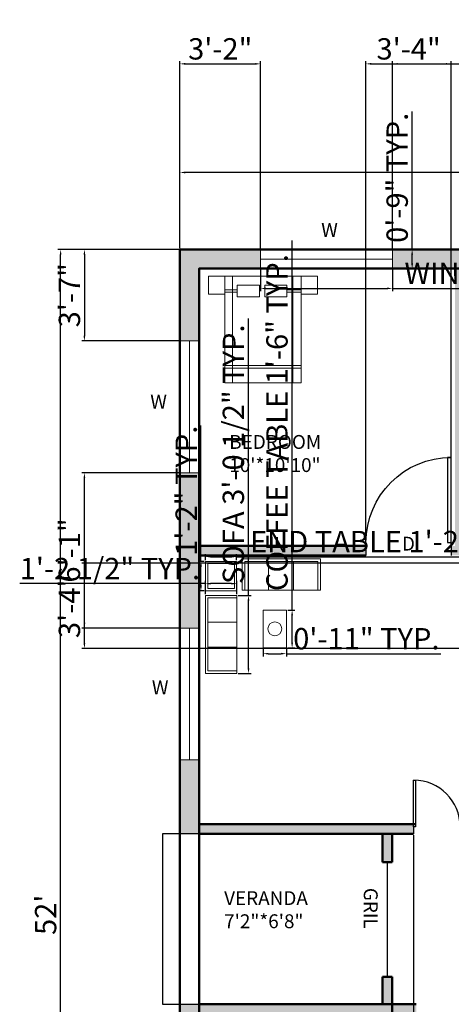
# Model space of a CAD drawing. Units: inches. Extents: x 1935 to 2445, y 1978 to 2806.
# Tile 2 of 4: x 1935 to 2137, y 2344 to 2806. Entities that reach past the tile are written whole.
import ezdxf

# ---------------------------------------------------------------- set-up
doc = ezdxf.new("R2010")
doc.units = ezdxf.units.IN
for name, color, linetype, lineweight in [('A-ANNO-DIMS', 2, 'Continuous', 18), ('A-ANNO-TEXT', 7, 'Continuous', 25), ('A-AREA-IDEN', 130, 'Continuous', 25), ('A-DOOR', 3, 'Continuous', 25), ('A-FLOR-GRIL', 3, 'Continuous', 25), ('A-FLOR-OTLN', 7, 'Continuous', 25), ('A-FURN', 9, 'Continuous', 18), ('A-GLAZ', 4, 'Continuous', 18), ('A-WALL-PATT', 225, 'Continuous', 13), ('SOFA', 10, 'Continuous', 18), ('WALL', 225, 'Continuous', 50)]:
    doc.layers.add(name, color=color, linetype=linetype, lineweight=lineweight)
doc.styles.get("Standard").update_dxf_attribs({"font": 'arial.ttf'})
doc.dimstyles.new('ISO-25', dxfattribs={"dimtxt": 10, "dimasz": 2.5, "dimexe": 1.25, "dimexo": 0.625, "dimtad": 1, "dimdec": 0, "dimlunit": 4, "dimtxsty": 'Standard', "dimcen": 2.5, "dimadec": 0, "dimazin": 0, "dimtfac": 1, "dimtdec": 0, "dimtmove": 0, "dimatfit": 3, "dimfxl": 1, "dimarcsym": 0})

# ---------------------------------------------------------------- blocks, each defined once
blk = doc.blocks.new('*U2')
for p, q in [((0, 0), (0, -6)), ((40, 0), (40, -6))]:
    blk.add_line(p, q)
blk.add_lwpolyline([(0, 0), (0, 40), (1.75, 40), (1.75, 0)], close=True)
blk.add_arc((0, 0), 40, 0, 90)
blk = doc.blocks.new('*D8')
at = {"layer": 'A-ANNO-DIMS', "color": 0, "lineweight": -2, "transparency": 16777216}
for p, q in [((2010.18, 2698.51), (2010.18, 2735.24)), ((2331.68, 2733.99), (2012.68, 2733.99)), ((2334.18, 2698.51), (2334.18, 2735.24))]:
    blk.add_line(p, q, dxfattribs=at)
at = {"layer": 'A-ANNO-DIMS', "color": 0, "lineweight": 100, "transparency": 16777216}
for points in [[(2012.68, 2734.4), (2012.68, 2733.57), (2010.18, 2733.99)], [(2331.68, 2734.4), (2331.68, 2733.57), (2334.18, 2733.99)]]:
    blk.add_solid(points, dxfattribs=at)
at = {"layer": 'Defpoints', "color": 0, "lineweight": 100, "transparency": 16777216}
for p in [(2010.18, 2733.99), (2010.18, 2697.88), (2334.18, 2697.88)]:
    blk.add_point(p, dxfattribs=at)
at = {"layer": 'A-ANNO-DIMS', "color": 0, "transparency": 16777216, "insert": (2172.18, 2739.63), "char_height": 10, "attachment_point": 5}
blk.add_mtext("27'", dxfattribs=at)
blk = doc.blocks.new('*D9')
at = {"layer": 'A-ANNO-DIMS', "color": 0, "lineweight": -2, "transparency": 16777216}
for p, q in [((2333.56, 2697.88), (1952.98, 2697.88)), ((1954.23, 2076.38), (1954.23, 2695.38)), ((2333.56, 2073.88), (1952.98, 2073.88))]:
    blk.add_line(p, q, dxfattribs=at)
at = {"layer": 'A-ANNO-DIMS', "color": 0, "lineweight": 100, "transparency": 16777216}
for points in [[(1953.82, 2695.38), (1954.65, 2695.38), (1954.23, 2697.88)], [(1953.82, 2076.38), (1954.65, 2076.38), (1954.23, 2073.88)]]:
    blk.add_solid(points, dxfattribs=at)
at = {"layer": 'Defpoints', "color": 0, "lineweight": 100, "transparency": 16777216}
for p in [(1954.23, 2697.88), (2334.18, 2697.88), (2334.18, 2073.88)]:
    blk.add_point(p, dxfattribs=at)
at = {"layer": 'A-ANNO-DIMS', "color": 0, "transparency": 16777216, "insert": (1948.5, 2385.88), "char_height": 10, "attachment_point": 5, "rotation": 90}
blk.add_mtext("52'", dxfattribs=at)
blk = doc.blocks.new('WINDOW-STD')
blk.add_line((0, 4.5), (61.82, 4.5))
blk.add_lwpolyline([(0, 9), (61.82, 9), (61.82, 0), (0, 0)], close=True)
blk = doc.blocks.new('BED-WITH-NIGHTSTANDS')
for p, q in [((11.32, 50.11), (11.32, 0)), ((39.64, 0), (39.64, 50.11)), ((13.46, 43.65), (7.73, 43.65)), ((13.46, 42.6), (7.73, 42.6)), ((43.47, 43.65), (36.85, 43.65)), ((43.47, 42.6), (36.85, 42.6)), ((7.73, 8.18), (43.47, 8.18)), ((7.73, 6.93), (43.47, 6.93)), ((43.47, 0), (39.64, 0))]:
    blk.add_line(p, q)
for points in [[(0, 50.11), (7.73, 50.11), (7.73, 41.64), (0, 41.64)], [(7.73, 50.11), (43.47, 50.11), (43.47, 0), (7.73, 0)], [(43.47, 50.11), (51.2, 50.11), (51.2, 41.64), (43.47, 41.64)], [(13.46, 45.91), (23.93, 45.91), (23.93, 40.33), (13.46, 40.33)], [(26.4, 45.91), (36.86, 45.91), (36.86, 40.33), (26.4, 40.33)]]:
    blk.add_lwpolyline(points, close=True)
blk = doc.blocks.new('SOFA-3-SEAT')
for p, q in [((0, 0), (0, 14.72)), ((0, 14.72), (36.65, 14.72)), ((36.65, 14.72), (36.65, 0)), ((12.37, 13.53), (12.37, 0)), ((24.09, 13.53), (24.09, 0)), ((1.26, 0), (0, 0)), ((36.65, 0), (31.67, 0))]:
    blk.add_line(p, q)
blk.add_lwpolyline([(1.26, 0), (35.43, 0), (35.43, 13.53), (1.26, 13.53)], close=True)
blk = doc.blocks.new('TABLE-END')
for points in [[(0, 13.76), (14.51, 13.76), (14.51, 0), (0, 0)], [(1, 12.76), (13.51, 12.76), (13.51, 1), (1, 1)]]:
    blk.add_lwpolyline(points, close=True)
blk = doc.blocks.new('TABLE-COFFEE')
blk.add_lwpolyline([(0, 0), (10.92, 0), (10.92, 17.81), (0, 17.81)], close=True)
blk.add_circle((5.5, 9), 3.27)
blk = doc.blocks.new('*D18')
at = {"layer": 'A-ANNO-DIMS', "color": 0, "lineweight": -2, "transparency": 16777216}
for p, q in [((2047.95, 2688.26), (2047.95, 2678.36)), ((2109.77, 2688.26), (2109.77, 2678.36)), ((2050.45, 2679.61), (2107.27, 2679.61)), ((2109.77, 2679.61), (2240.06, 2679.61))]:
    blk.add_line(p, q, dxfattribs=at)
at = {"layer": 'A-ANNO-DIMS', "color": 0, "lineweight": 100, "transparency": 16777216}
for points in [[(2050.45, 2680.03), (2050.45, 2679.19), (2047.95, 2679.61)], [(2107.27, 2680.03), (2107.27, 2679.19), (2109.77, 2679.61)]]:
    blk.add_solid(points, dxfattribs=at)
at = {"layer": 'Defpoints', "color": 0, "lineweight": 100, "transparency": 16777216}
for p in [(2047.95, 2688.88), (2109.77, 2688.88), (2109.77, 2679.61)]:
    blk.add_point(p, dxfattribs=at)
at = {"layer": 'A-ANNO-DIMS', "color": 0, "transparency": 16777216, "insert": (2176.16, 2685.41), "char_height": 10, "attachment_point": 5}
blk.add_mtext('WINDOW 5\'-2" TYP.', dxfattribs=at)
blk = doc.blocks.new('*D19')
at = {"layer": 'A-ANNO-DIMS', "color": 0, "lineweight": -2, "transparency": 16777216}
for p, q in [((2119.04, 2697.88), (2119.04, 2762.59)), ((2110.39, 2697.88), (2120.29, 2697.88)), ((2119.04, 2691.38), (2119.04, 2695.38)), ((2110.39, 2688.88), (2120.29, 2688.88))]:
    blk.add_line(p, q, dxfattribs=at)
at = {"layer": 'A-ANNO-DIMS', "color": 0, "lineweight": 100, "transparency": 16777216}
for points in [[(2118.62, 2695.38), (2119.46, 2695.38), (2119.04, 2697.88)], [(2118.62, 2691.38), (2119.46, 2691.38), (2119.04, 2688.88)]]:
    blk.add_solid(points, dxfattribs=at)
at = {"layer": 'Defpoints', "color": 0, "lineweight": 100, "transparency": 16777216}
for p in [(2109.77, 2697.88), (2119.04, 2697.88), (2109.77, 2688.88)]:
    blk.add_point(p, dxfattribs=at)
at = {"layer": 'A-ANNO-DIMS', "color": 0, "transparency": 16777216, "insert": (2113.31, 2731.49), "char_height": 10, "attachment_point": 5, "rotation": 90}
blk.add_mtext('0\'-9" TYP.', dxfattribs=at)
blk = doc.blocks.new('*D24')
at = {"layer": 'A-ANNO-DIMS', "color": 0, "lineweight": -2, "transparency": 16777216}
for p, q in [((2042.32, 2535.66), (2042.32, 2665.53)), ((2037.44, 2535.66), (2043.57, 2535.66)), ((2042.32, 2501.51), (2042.32, 2533.16)), ((2037.44, 2499.01), (2043.57, 2499.01))]:
    blk.add_line(p, q, dxfattribs=at)
at = {"layer": 'A-ANNO-DIMS', "color": 0, "lineweight": 100, "transparency": 16777216}
for points in [[(2041.9, 2533.16), (2042.73, 2533.16), (2042.32, 2535.66)], [(2041.9, 2501.51), (2042.73, 2501.51), (2042.32, 2499.01)]]:
    blk.add_solid(points, dxfattribs=at)
at = {"layer": 'Defpoints', "color": 0, "lineweight": 100, "transparency": 16777216}
for p in [(2036.82, 2535.66), (2042.32, 2535.66), (2036.82, 2499.01)]:
    blk.add_point(p, dxfattribs=at)
at = {"layer": 'A-ANNO-DIMS', "color": 0, "transparency": 16777216, "insert": (2036.51, 2601.85), "char_height": 10, "attachment_point": 5, "rotation": 90}
blk.add_mtext('SOFA 3\'-0 1/2" TYP.', dxfattribs=at)
blk = doc.blocks.new('*D25')
at = {"layer": 'A-ANNO-DIMS', "color": 0, "lineweight": -2, "transparency": 16777216}
for p, q in [((2022.1, 2541.16), (1935.04, 2541.16)), ((2022.1, 2536.28), (2022.1, 2542.41)), ((2034.32, 2541.16), (2024.6, 2541.16)), ((2036.82, 2536.28), (2036.82, 2542.41))]:
    blk.add_line(p, q, dxfattribs=at)
at = {"layer": 'A-ANNO-DIMS', "color": 0, "lineweight": 100, "transparency": 16777216}
for points in [[(2024.6, 2541.57), (2024.6, 2540.74), (2022.1, 2541.16)], [(2034.32, 2541.57), (2034.32, 2540.74), (2036.82, 2541.16)]]:
    blk.add_solid(points, dxfattribs=at)
at = {"layer": 'Defpoints', "color": 0, "lineweight": 100, "transparency": 16777216}
for p in [(2022.1, 2541.16), (2022.1, 2535.66), (2036.82, 2535.66)]:
    blk.add_point(p, dxfattribs=at)
at = {"layer": 'A-ANNO-DIMS', "color": 0, "transparency": 16777216, "insert": (1977.32, 2546.95), "char_height": 10, "attachment_point": 5}
blk.add_mtext('1\'-2 1/2" TYP.', dxfattribs=at)
blk = doc.blocks.new('*D26')
at = {"layer": 'A-ANNO-DIMS', "color": 0, "lineweight": -2, "transparency": 16777216}
for p, q in [((2022.21, 2552.24), (2022.21, 2555.04)), ((2024.71, 2553.79), (2034.22, 2553.79)), ((2036.72, 2552.24), (2036.72, 2555.04)), ((2036.72, 2553.79), (2205.72, 2553.79))]:
    blk.add_line(p, q, dxfattribs=at)
at = {"layer": 'A-ANNO-DIMS', "color": 0, "lineweight": 100, "transparency": 16777216}
for points in [[(2024.71, 2554.21), (2024.71, 2553.37), (2022.21, 2553.79)], [(2034.22, 2554.21), (2034.22, 2553.37), (2036.72, 2553.79)]]:
    blk.add_solid(points, dxfattribs=at)
at = {"layer": 'Defpoints', "color": 0, "lineweight": 100, "transparency": 16777216}
for p in [(2036.72, 2553.79), (2022.21, 2551.61), (2036.72, 2551.61)]:
    blk.add_point(p, dxfattribs=at)
at = {"layer": 'A-ANNO-DIMS', "color": 0, "transparency": 16777216, "insert": (2122.47, 2559.59), "char_height": 10, "attachment_point": 5}
blk.add_mtext('END TABLE 1\'-2 1/2" TYP.', dxfattribs=at)
blk = doc.blocks.new('*D27')
at = {"layer": 'A-ANNO-DIMS', "color": 0, "lineweight": -2, "transparency": 16777216}
for p, q in [((2020.04, 2551.61), (2020.04, 2615.38)), ((2021.59, 2551.61), (2018.79, 2551.61)), ((2020.04, 2540.35), (2020.04, 2549.11)), ((2021.59, 2537.85), (2018.79, 2537.85))]:
    blk.add_line(p, q, dxfattribs=at)
at = {"layer": 'A-ANNO-DIMS', "color": 0, "lineweight": 100, "transparency": 16777216}
for points in [[(2019.62, 2549.11), (2020.46, 2549.11), (2020.04, 2551.61)], [(2019.62, 2540.35), (2020.46, 2540.35), (2020.04, 2537.85)]]:
    blk.add_solid(points, dxfattribs=at)
at = {"layer": 'Defpoints', "color": 0, "lineweight": 100, "transparency": 16777216}
for p in [(2020.04, 2551.61), (2022.21, 2551.61), (2022.21, 2537.85)]:
    blk.add_point(p, dxfattribs=at)
at = {"layer": 'A-ANNO-DIMS', "color": 0, "transparency": 16777216, "insert": (2014.39, 2584.75), "char_height": 10, "attachment_point": 5, "rotation": 90}
blk.add_mtext('1\'-2" TYP.', dxfattribs=at)
blk = doc.blocks.new('*D28')
at = {"layer": 'A-ANNO-DIMS', "color": 0, "lineweight": -2, "transparency": 16777216}
for p, q in [((2062.76, 2528.8), (2062.76, 2702.06)), ((2060.71, 2528.8), (2064.01, 2528.8)), ((2062.76, 2513.49), (2062.76, 2526.3)), ((2060.71, 2510.99), (2064.01, 2510.99))]:
    blk.add_line(p, q, dxfattribs=at)
at = {"layer": 'A-ANNO-DIMS', "color": 0, "lineweight": 100, "transparency": 16777216}
for points in [[(2062.34, 2526.3), (2063.17, 2526.3), (2062.76, 2528.8)], [(2062.34, 2513.49), (2063.17, 2513.49), (2062.76, 2510.99)]]:
    blk.add_solid(points, dxfattribs=at)
at = {"layer": 'Defpoints', "color": 0, "lineweight": 100, "transparency": 16777216}
for p in [(2060.08, 2528.8), (2062.76, 2528.8), (2060.08, 2510.99)]:
    blk.add_point(p, dxfattribs=at)
at = {"layer": 'A-ANNO-DIMS', "color": 0, "transparency": 16777216, "insert": (2056.96, 2616.68), "char_height": 10, "attachment_point": 5, "rotation": 90}
blk.add_mtext('COFFEE TABLE 1\'-6" TYP.', dxfattribs=at)
blk = doc.blocks.new('*D29')
at = {"layer": 'A-ANNO-DIMS', "color": 0, "lineweight": -2, "transparency": 16777216}
for p, q in [((2049.17, 2510.36), (2049.17, 2507.07)), ((2051.67, 2508.32), (2057.58, 2508.32)), ((2060.08, 2510.36), (2060.08, 2507.07)), ((2060.08, 2508.32), (2132.56, 2508.32))]:
    blk.add_line(p, q, dxfattribs=at)
at = {"layer": 'A-ANNO-DIMS', "color": 0, "lineweight": 100, "transparency": 16777216}
for points in [[(2051.67, 2508.73), (2051.67, 2507.9), (2049.17, 2508.32)], [(2057.58, 2508.73), (2057.58, 2507.9), (2060.08, 2508.32)]]:
    blk.add_solid(points, dxfattribs=at)
at = {"layer": 'Defpoints', "color": 0, "lineweight": 100, "transparency": 16777216}
for p in [(2049.17, 2510.99), (2060.08, 2510.99), (2060.08, 2508.32)]:
    blk.add_point(p, dxfattribs=at)
at = {"layer": 'A-ANNO-DIMS', "color": 0, "transparency": 16777216, "insert": (2097.57, 2514.05), "char_height": 10, "attachment_point": 5}
blk.add_mtext('0\'-11" TYP.', dxfattribs=at)
blk = doc.blocks.new('*D34')
at = {"layer": 'A-ANNO-DIMS', "color": 0, "lineweight": -2, "transparency": 16777216}
for p, q in [((2010.18, 2698.51), (2010.18, 2786.17)), ((2012.68, 2784.92), (2045.45, 2784.92)), ((2047.95, 2698.51), (2047.95, 2786.17))]:
    blk.add_line(p, q, dxfattribs=at)
at = {"layer": 'A-ANNO-DIMS', "color": 0, "lineweight": 100, "transparency": 16777216}
for points in [[(2012.68, 2785.34), (2012.68, 2784.51), (2010.18, 2784.92)], [(2045.45, 2785.34), (2045.45, 2784.51), (2047.95, 2784.92)]]:
    blk.add_solid(points, dxfattribs=at)
at = {"layer": 'Defpoints', "color": 0, "lineweight": 100, "transparency": 16777216}
for p in [(2047.95, 2784.92), (2010.18, 2697.88), (2047.95, 2697.88)]:
    blk.add_point(p, dxfattribs=at)
at = {"layer": 'A-ANNO-DIMS', "color": 0, "transparency": 16777216, "insert": (2029.07, 2790.66), "char_height": 10, "attachment_point": 5}
blk.add_mtext('3\'-2"', dxfattribs=at)
blk = doc.blocks.new('*D35')
at = {"layer": 'A-ANNO-DIMS', "color": 0, "lineweight": -2, "transparency": 16777216}
for p, q in [((2109.77, 2698.51), (2109.77, 2786.17)), ((2112.27, 2784.92), (2153.67, 2784.92)), ((2156.17, 2698.51), (2156.17, 2786.17)), ((2156.17, 2784.92), (2217.57, 2784.92))]:
    blk.add_line(p, q, dxfattribs=at)
at = {"layer": 'A-ANNO-DIMS', "color": 0, "lineweight": 100, "transparency": 16777216}
for points in [[(2112.27, 2785.34), (2112.27, 2784.51), (2109.77, 2784.92)], [(2153.67, 2785.34), (2153.67, 2784.51), (2156.17, 2784.92)]]:
    blk.add_solid(points, dxfattribs=at)
at = {"layer": 'Defpoints', "color": 0, "lineweight": 100, "transparency": 16777216}
for p in [(2156.17, 2784.92), (2109.77, 2697.88), (2156.17, 2697.88)]:
    blk.add_point(p, dxfattribs=at)
at = {"layer": 'A-ANNO-DIMS', "color": 0, "transparency": 16777216, "insert": (2188.12, 2790.72), "char_height": 10, "attachment_point": 5}
blk.add_mtext('3\'-10 1/2"', dxfattribs=at)
blk = doc.blocks.new('*D37')
at = {"layer": 'A-ANNO-DIMS', "color": 0, "lineweight": -2, "transparency": 16777216}
for p, q in [((2009.56, 2697.88), (1964.13, 2697.88)), ((1965.38, 2695.38), (1965.38, 2657.46)), ((2009.56, 2654.96), (1964.13, 2654.96))]:
    blk.add_line(p, q, dxfattribs=at)
at = {"layer": 'A-ANNO-DIMS', "color": 0, "lineweight": 100, "transparency": 16777216}
for points in [[(1964.96, 2695.38), (1965.8, 2695.38), (1965.38, 2697.88)], [(1964.96, 2657.46), (1965.8, 2657.46), (1965.38, 2654.96)]]:
    blk.add_solid(points, dxfattribs=at)
at = {"layer": 'Defpoints', "color": 0, "lineweight": 100, "transparency": 16777216}
for p in [(2010.18, 2697.88), (1965.38, 2654.96), (2010.18, 2654.96)]:
    blk.add_point(p, dxfattribs=at)
at = {"layer": 'A-ANNO-DIMS', "color": 0, "transparency": 16777216, "insert": (1959.65, 2676.42), "char_height": 10, "attachment_point": 5, "rotation": 90}
blk.add_mtext('3\'-7"', dxfattribs=at)
blk = doc.blocks.new('*D38')
at = {"layer": 'A-ANNO-DIMS', "color": 0, "lineweight": -2, "transparency": 16777216}
for p, q in [((2009.56, 2593.14), (1964.13, 2593.14)), ((1965.38, 2522.81), (1965.38, 2590.64)), ((2009.56, 2520.31), (1964.13, 2520.31))]:
    blk.add_line(p, q, dxfattribs=at)
at = {"layer": 'A-ANNO-DIMS', "color": 0, "lineweight": 100, "transparency": 16777216}
for points in [[(1964.96, 2590.64), (1965.8, 2590.64), (1965.38, 2593.14)], [(1964.96, 2522.81), (1965.8, 2522.81), (1965.38, 2520.31)]]:
    blk.add_solid(points, dxfattribs=at)
at = {"layer": 'Defpoints', "color": 0, "lineweight": 100, "transparency": 16777216}
for p in [(1965.38, 2593.14), (2010.18, 2593.14), (2010.18, 2520.31)]:
    blk.add_point(p, dxfattribs=at)
at = {"layer": 'A-ANNO-DIMS', "color": 0, "transparency": 16777216, "insert": (1959.65, 2556.72), "char_height": 10, "attachment_point": 5, "rotation": 90}
blk.add_mtext('6\'-1"', dxfattribs=at)
blk = doc.blocks.new('*D39')
at = {"layer": 'A-ANNO-DIMS', "color": 0, "lineweight": -2, "transparency": 16777216}
for p, q in [((2019.18, 2423.26), (2019.18, 1986.08)), ((2119.73, 2423.26), (2119.73, 1986.08)), ((2021.68, 1987.33), (2117.23, 1987.33))]:
    blk.add_line(p, q, dxfattribs=at)
at = {"layer": 'A-ANNO-DIMS', "color": 0, "lineweight": 100, "transparency": 16777216}
for points in [[(2021.68, 1987.74), (2021.68, 1986.91), (2019.18, 1987.33)], [(2117.23, 1987.74), (2117.23, 1986.91), (2119.73, 1987.33)]]:
    blk.add_solid(points, dxfattribs=at)
at = {"layer": 'Defpoints', "color": 0, "lineweight": 100, "transparency": 16777216}
for p in [(2019.18, 2423.88), (2119.73, 2423.88), (2119.73, 1987.33)]:
    blk.add_point(p, dxfattribs=at)
at = {"layer": 'A-ANNO-DIMS', "color": 0, "transparency": 16777216, "insert": (2069.46, 1993.12), "char_height": 10, "attachment_point": 5}
blk.add_mtext('8\'-4 1/2"', dxfattribs=at)
blk = doc.blocks.new('*D40')
at = {"layer": 'A-ANNO-DIMS', "color": 0, "lineweight": -2, "transparency": 16777216}
for p, q in [((2119.73, 2423.26), (2119.73, 1986.08)), ((2163.45, 2423.26), (2163.45, 1986.08)), ((2122.23, 1987.33), (2160.95, 1987.33)), ((2163.45, 1987.33), (2217.08, 1987.33))]:
    blk.add_line(p, q, dxfattribs=at)
at = {"layer": 'A-ANNO-DIMS', "color": 0, "lineweight": 100, "transparency": 16777216}
for points in [[(2122.23, 1987.74), (2122.23, 1986.91), (2119.73, 1987.33)], [(2160.95, 1987.74), (2160.95, 1986.91), (2163.45, 1987.33)]]:
    blk.add_solid(points, dxfattribs=at)
at = {"layer": 'Defpoints', "color": 0, "lineweight": 100, "transparency": 16777216}
for p in [(2119.73, 2423.88), (2163.45, 2423.88), (2163.45, 1987.33)]:
    blk.add_point(p, dxfattribs=at)
at = {"layer": 'A-ANNO-DIMS', "color": 0, "transparency": 16777216, "insert": (2191.52, 1993.13), "char_height": 10, "attachment_point": 5}
blk.add_mtext('3\'-7 1/2"', dxfattribs=at)
blk = doc.blocks.new('*D41')
at = {"layer": 'A-ANNO-DIMS', "color": 0, "lineweight": -2, "transparency": 16777216}
for p, q in [((2097.4, 2559.51), (2097.4, 2786.17)), ((2099.9, 2784.92), (2134.9, 2784.92)), ((2137.4, 2559.51), (2137.4, 2786.17))]:
    blk.add_line(p, q, dxfattribs=at)
at = {"layer": 'A-ANNO-DIMS', "color": 0, "lineweight": 100, "transparency": 16777216}
for points in [[(2099.9, 2785.34), (2099.9, 2784.51), (2097.4, 2784.92)], [(2134.9, 2785.34), (2134.9, 2784.51), (2137.4, 2784.92)]]:
    blk.add_solid(points, dxfattribs=at)
at = {"layer": 'Defpoints', "color": 0, "lineweight": 100, "transparency": 16777216}
for p in [(2137.4, 2784.92), (2097.4, 2558.88), (2137.4, 2558.88)]:
    blk.add_point(p, dxfattribs=at)
at = {"layer": 'A-ANNO-DIMS', "color": 0, "transparency": 16777216, "insert": (2117.4, 2790.66), "char_height": 10, "attachment_point": 5}
blk.add_mtext('3\'-4"', dxfattribs=at)
blk = doc.blocks.new('*D43')
at = {"layer": 'A-ANNO-DIMS', "color": 0, "lineweight": -2, "transparency": 16777216}
for p, q in [((2242.06, 2550.71), (1964.13, 2550.71)), ((1965.38, 2513.21), (1965.38, 2548.21)), ((2242.06, 2510.71), (1964.13, 2510.71))]:
    blk.add_line(p, q, dxfattribs=at)
at = {"layer": 'A-ANNO-DIMS', "color": 0, "lineweight": 100, "transparency": 16777216}
for points in [[(1964.96, 2548.21), (1965.8, 2548.21), (1965.38, 2550.71)], [(1964.96, 2513.21), (1965.8, 2513.21), (1965.38, 2510.71)]]:
    blk.add_solid(points, dxfattribs=at)
at = {"layer": 'Defpoints', "color": 0, "lineweight": 100, "transparency": 16777216}
for p in [(1965.38, 2550.71), (2242.68, 2550.71), (2242.68, 2510.71)]:
    blk.add_point(p, dxfattribs=at)
at = {"layer": 'A-ANNO-DIMS', "color": 0, "transparency": 16777216, "insert": (1959.65, 2530.71), "char_height": 10, "attachment_point": 5, "rotation": 90}
blk.add_mtext('3\'-4"', dxfattribs=at)

msp = doc.modelspace()

# ---------------------------------------------------------------- hatches: boundary and pattern name
at = {"layer": 'A-WALL-PATT'}
h = msp.add_hatch(color=256, dxfattribs=at)
h.dxf.hatch_style = 1
h.paths.add_polyline_path([(2047.95, 2697.88), (2010.18, 2697.88), (2010.18, 2654.96), (2019.18, 2654.96), (2019.18, 2688.88), (2047.95, 2688.88)], flags=16)
h.paths.add_polyline_path([(2156.17, 2697.88), (2109.77, 2697.88), (2109.77, 2688.88), (2139.18, 2688.88), (2156.17, 2688.88)], flags=17)
h.paths.add_polyline_path([(2231.53, 2697.88), (2186.46, 2697.88), (2186.46, 2688.88), (2231.53, 2688.88)], flags=17)
h.paths.add_polyline_path([(2334.18, 2697.88), (2293.35, 2697.88), (2293.35, 2688.88), (2325.18, 2688.88), (2325.18, 2651.52), (2334.18, 2651.52)], flags=17)
h.paths.add_polyline_path([(2247.18, 2554.38), (2242.68, 2554.38), (2242.68, 2550.71), (2247.18, 2550.71)], flags=17)
h.paths.add_polyline_path([(2145.55, 2592.49), (2145.55, 2592.88), (2143.68, 2592.88), (2143.68, 2588.39), (2145.55, 2588.39)], flags=17)
h.paths.add_polyline_path([(2197.68, 2592.88), (2172.86, 2592.88, -0.003651), (2172.86, 2592.49), (2172.86, 2588.39), (2197.68, 2588.39)], flags=17)
h.paths.add_polyline_path([(2203.16, 2558.88), (2137.4, 2558.88), (2137.4, 2554.38), (2143.68, 2554.38), (2203.16, 2554.38)], flags=17)
h.paths.add_polyline_path([(2097.4, 2558.88), (2019.18, 2558.88), (2019.18, 2554.38), (2097.4, 2554.38)], flags=17)
h.paths.add_polyline_path([(2143.68, 2688.88), (2139.18, 2688.88), (2139.18, 2558.88), (2143.68, 2558.88)], flags=17)
h.paths.add_polyline_path([(2202.18, 2688.88), (2197.68, 2688.88), (2197.68, 2592.88), (2197.68, 2588.39), (2197.68, 2558.88), (2202.18, 2558.88), (2202.18, 2588.38)], flags=17)
h.paths.add_polyline_path([(2241.74, 2229.79), (2251.55, 2229.79), (2251.55, 2243.19), (2241.74, 2243.19)], flags=25)
h.paths.add_polyline_path([(2215.53, 2200.14), (2225.34, 2200.14), (2225.34, 2213.54), (2215.53, 2213.54)], flags=25)
h.paths.add_polyline_path([(2152.61, 2173.98), (2162.42, 2173.98), (2162.42, 2187.38), (2152.61, 2187.38)], flags=25)
h.paths.add_polyline_path([(2109.99, 2200.78), (2119.8, 2200.78), (2119.8, 2214.18), (2109.99, 2214.18)], flags=25)
h.paths.add_polyline_path([(2139.65, 2343.23), (2149.46, 2343.23), (2149.46, 2356.63), (2139.65, 2356.63)], flags=25)
h.paths.add_polyline_path([(2138.05, 2412.22), (2147.87, 2412.22), (2147.87, 2425.62), (2138.05, 2425.62)], flags=25)
h.paths.add_polyline_path([(2242.1, 2526.57), (2251.91, 2526.57), (2251.91, 2539.97), (2242.1, 2539.97)], flags=25)
h.paths.add_polyline_path([(2212.92, 2555.35), (2222.74, 2555.35), (2222.74, 2568.75), (2212.92, 2568.75)], flags=25)
h.paths.add_polyline_path([(2111.94, 2553.1), (2121.75, 2553.1), (2121.75, 2566.5), (2111.94, 2566.5)], flags=25)
h.paths.add_polyline_path([(2032.85, 2161.17), (2083.36, 2161.17), (2083.36, 2185.43), (2032.85, 2185.43)], flags=25)
h.paths.add_polyline_path([(2145.49, 2119.25), (2193.41, 2119.25), (2193.41, 2143.52), (2145.49, 2143.52)], flags=25)
h.paths.add_polyline_path([(2250.93, 2163.1), (2301.44, 2163.1), (2301.44, 2187.36), (2250.93, 2187.36)], flags=25)
h.paths.add_polyline_path([(2247.75, 2274.43), (2290.88, 2274.43), (2290.88, 2298.69), (2247.75, 2298.69)], flags=25)
h.paths.add_polyline_path([(2131.26, 2265.2), (2178.71, 2265.2), (2178.71, 2289.46), (2131.26, 2289.46)], flags=25)
h.paths.add_polyline_path([(2092.71, 2400.61), (2092.71, 2376.16), (2106.11, 2376.16), (2106.11, 2400.61)], flags=25)
h.paths.add_polyline_path([(2173.61, 2396.23), (2189.48, 2396.23), (2189.48, 2409.63), (2173.61, 2409.63)], flags=25)
h.paths.add_polyline_path([(2028.85, 2376.01), (2076.42, 2376.01), (2076.42, 2400.28), (2028.85, 2400.28)], flags=25)
h.paths.add_polyline_path([(2135.3, 2481.1), (2182.75, 2481.1), (2182.75, 2505.37), (2135.3, 2505.37)], flags=25)
h.paths.add_polyline_path([(2249.01, 2476.21), (2292.13, 2476.21), (2292.13, 2500.47), (2249.01, 2500.47)], flags=25)
h.paths.add_polyline_path([(2251.9, 2596.84), (2302.42, 2596.84), (2302.42, 2621.11), (2251.9, 2621.11)], flags=25)
h.paths.add_polyline_path([(2030.66, 2589.83), (2081.18, 2589.83), (2081.18, 2614.09), (2030.66, 2614.09)], flags=25)
h.paths.add_polyline_path([(2019.18, 2593.14), (2010.18, 2593.14), (2010.18, 2520.31), (2019.18, 2520.31)])
h.paths.add_polyline_path([(2010.18, 2164.99), (2019.18, 2164.99), (2019.18, 2238.56), (2010.18, 2238.56)])
h.paths.add_polyline_path([(2048.33, 2073.88), (2048.33, 2082.88), (2019.18, 2082.88), (2019.18, 2103.18), (2010.18, 2103.18), (2010.18, 2073.88)])
h.paths.add_polyline_path([(2156.55, 2073.88), (2156.55, 2082.88), (2110.15, 2082.88), (2110.15, 2073.88)])
h.paths.add_polyline_path([(2231.91, 2073.88), (2231.91, 2082.88), (2186.84, 2082.88), (2186.84, 2073.88)])
h.paths.add_polyline_path([(2047.95, 2688.88), (2047.95, 2697.88), (2010.18, 2697.88), (2010.18, 2654.96), (2019.18, 2654.96), (2019.18, 2688.88)])
h.paths.add_polyline_path([(2109.77, 2697.88), (2109.77, 2688.88), (2156.17, 2688.88), (2156.17, 2697.88)])
h = msp.add_hatch(color=256, dxfattribs=at)
h.dxf.hatch_style = 1
h.paths.add_polyline_path([(2196.68, 2183.38), (2171.78, 2183.38), (2171.78, 2179.29, -0.003687), (2171.78, 2178.88), (2196.68, 2178.88)], flags=17)
h.paths.add_polyline_path([(2144.47, 2183.38), (2142.68, 2183.38), (2142.68, 2178.88), (2144.47, 2178.88), (2144.47, 2179.29)], flags=17)
h.paths.add_polyline_path([(2096.62, 2213.38), (2019.18, 2213.38), (2019.18, 2208.88), (2096.62, 2208.88)], flags=17)
h.paths.add_polyline_path([(2142.68, 2208.88), (2142.68, 2213.38), (2136.62, 2213.38), (2136.62, 2208.88), (2138.18, 2208.88), (2138.18, 2183.38), (2138.18, 2082.88), (2142.68, 2082.88), (2142.68, 2178.88), (2142.68, 2183.38)], flags=17)
h.paths.add_polyline_path([(2201.18, 2208.88), (2202.06, 2208.88), (2202.06, 2213.38), (2196.68, 2213.38), (2196.68, 2204.97), (2196.68, 2082.88), (2201.18, 2082.88)], flags=17)
h.paths.add_polyline_path([(2247.18, 2217.21), (2242.68, 2217.21), (2242.68, 2213.38), (2247.18, 2213.38)], flags=17)
h.paths.add_polyline_path([(2325.18, 2213.38), (2242.68, 2213.38), (2242.68, 2208.88), (2325.18, 2208.88)], flags=17)
h.paths.add_polyline_path([(2247.18, 2339.38), (2242.68, 2339.38), (2242.68, 2257.21), (2247.18, 2257.21)], flags=17)
h.paths.add_polyline_path([(2325.18, 2343.88), (2286.18, 2343.88), (2186.18, 2343.88), (2164.69, 2343.88), (2164.69, 2340.61), (2164.69, 2339.38), (2213.9, 2339.38), (2286.18, 2339.38), (2325.18, 2339.38)], flags=17)
h.paths.add_polyline_path([(2109.68, 2343.88), (2105.18, 2343.88), (2019.18, 2343.88), (2019.18, 2339.38), (2109.68, 2339.38)], flags=17)
h.paths.add_polyline_path([(2120.97, 2340.61), (2120.97, 2343.88), (2109.68, 2343.88), (2109.68, 2339.38), (2120.97, 2339.38)], flags=17)
h.paths.add_polyline_path([(2109.68, 2356.84), (2105.18, 2356.84), (2105.18, 2343.88), (2109.68, 2343.88)], flags=17)
h.paths.add_polyline_path([(2230.51, 2409.48), (2245.95, 2409.48), (2245.95, 2430.09), (2230.51, 2430.09)], flags=25)
h.paths.add_polyline_path([(2289.31, 2409.69), (2322.13, 2409.69), (2322.13, 2430.3), (2289.31, 2430.3)], flags=25)
h.paths.add_polyline_path([(2241.74, 2229.79), (2251.55, 2229.79), (2251.55, 2243.19), (2241.74, 2243.19)], flags=25)
h.paths.add_polyline_path([(2215.53, 2200.14), (2225.34, 2200.14), (2225.34, 2213.54), (2215.53, 2213.54)], flags=25)
h.paths.add_polyline_path([(2152.61, 2173.98), (2162.42, 2173.98), (2162.42, 2187.38), (2152.61, 2187.38)], flags=25)
h.paths.add_polyline_path([(2109.99, 2200.78), (2119.8, 2200.78), (2119.8, 2214.18), (2109.99, 2214.18)], flags=25)
h.paths.add_polyline_path([(2139.65, 2343.23), (2149.46, 2343.23), (2149.46, 2356.63), (2139.65, 2356.63)], flags=25)
h.paths.add_polyline_path([(2138.05, 2412.22), (2147.87, 2412.22), (2147.87, 2425.62), (2138.05, 2425.62)], flags=25)
h.paths.add_polyline_path([(2242.1, 2526.57), (2251.91, 2526.57), (2251.91, 2539.97), (2242.1, 2539.97)], flags=25)
h.paths.add_polyline_path([(2212.92, 2555.35), (2222.74, 2555.35), (2222.74, 2568.75), (2212.92, 2568.75)], flags=25)
h.paths.add_polyline_path([(2151.96, 2587.49), (2161.77, 2587.49), (2161.77, 2600.89), (2151.96, 2600.89)], flags=25)
h.paths.add_polyline_path([(2111.94, 2553.1), (2121.75, 2553.1), (2121.75, 2566.5), (2111.94, 2566.5)], flags=25)
h.paths.add_polyline_path([(2032.85, 2161.17), (2083.36, 2161.17), (2083.36, 2185.43), (2032.85, 2185.43)], flags=25)
h.paths.add_polyline_path([(2145.49, 2119.25), (2193.41, 2119.25), (2193.41, 2143.52), (2145.49, 2143.52)], flags=25)
h.paths.add_polyline_path([(2250.93, 2163.1), (2301.44, 2163.1), (2301.44, 2187.36), (2250.93, 2187.36)], flags=25)
h.paths.add_polyline_path([(2247.75, 2274.43), (2290.88, 2274.43), (2290.88, 2298.69), (2247.75, 2298.69)], flags=25)
h.paths.add_polyline_path([(2131.26, 2265.2), (2178.71, 2265.2), (2178.71, 2289.46), (2131.26, 2289.46)], flags=25)
h.paths.add_polyline_path([(2173.61, 2396.23), (2189.48, 2396.23), (2189.48, 2409.63), (2173.61, 2409.63)], flags=25)
h.paths.add_polyline_path([(2135.3, 2481.1), (2182.75, 2481.1), (2182.75, 2505.37), (2135.3, 2505.37)], flags=25)
h.paths.add_polyline_path([(2249.01, 2476.21), (2292.13, 2476.21), (2292.13, 2500.47), (2249.01, 2500.47)], flags=25)
h.paths.add_polyline_path([(2251.9, 2596.84), (2302.42, 2596.84), (2302.42, 2621.11), (2251.9, 2621.11)], flags=25)
h.paths.add_polyline_path([(2148.05, 2628.52), (2195.98, 2628.52), (2195.98, 2652.78), (2148.05, 2652.78)], flags=25)
h.paths.add_polyline_path([(2030.66, 2589.83), (2081.18, 2589.83), (2081.18, 2614.09), (2030.66, 2614.09)], flags=25)
h.paths.add_polyline_path([(2325.18, 2414.18), (2334.18, 2414.18), (2334.18, 2455.16), (2325.18, 2455.16)])
h.paths.add_polyline_path([(2325.18, 2305.65), (2334.18, 2305.65), (2334.18, 2352.36), (2325.18, 2352.36)])
h.paths.add_polyline_path([(2325.18, 2163.2), (2334.18, 2163.2), (2334.18, 2243.83), (2325.18, 2243.83)])
h.paths.add_polyline_path([(2293.73, 2082.88), (2293.73, 2073.88), (2334.18, 2073.88), (2334.18, 2101.39), (2325.18, 2101.39), (2325.18, 2082.88)])
h.paths.add_polyline_path([(2334.18, 2589.71), (2325.18, 2589.71), (2325.18, 2516.98), (2334.18, 2516.98)])
h.paths.add_polyline_path([(2293.35, 2697.88), (2293.35, 2688.88), (2325.18, 2688.88), (2325.18, 2651.52), (2334.18, 2651.52), (2334.18, 2697.88)])
h.paths.add_polyline_path([(2109.77, 2697.88), (2109.77, 2688.88), (2231.53, 2688.88), (2231.53, 2697.88)])
h.paths.add_polyline_path([(2010.18, 2654.96), (2019.18, 2654.96), (2019.18, 2688.88), (2047.95, 2688.88), (2047.95, 2697.88), (2010.18, 2697.88)])
h.paths.add_polyline_path([(2010.18, 2520.31), (2019.18, 2520.31), (2019.18, 2593.14), (2010.18, 2593.14)])
h = msp.add_hatch(color=256, dxfattribs=at)
h.dxf.hatch_style = 1
h.paths.add_polyline_path([(2334.18, 2589.71), (2325.18, 2589.71), (2325.18, 2516.98), (2334.18, 2516.98)])
h.paths.add_polyline_path([(2325.18, 2558.88), (2240.84, 2558.88), (2240.84, 2554.38), (2325.18, 2554.38)])
h.paths.add_polyline_path([(2119.73, 2427.16), (2119.73, 2428.38), (2019.18, 2428.38), (2019.18, 2423.88), (2119.73, 2423.88)])
h.paths.add_polyline_path([(2230.51, 2409.48), (2245.95, 2409.48), (2245.95, 2430.09), (2230.51, 2430.09)], flags=9)
h.paths.add_polyline_path([(2289.31, 2409.69), (2322.13, 2409.69), (2322.13, 2430.3), (2289.31, 2430.3)], flags=9)
h.paths.add_polyline_path([(2241.74, 2229.79), (2251.55, 2229.79), (2251.55, 2243.19), (2241.74, 2243.19)], flags=9)
h.paths.add_polyline_path([(2215.53, 2200.14), (2225.34, 2200.14), (2225.34, 2213.54), (2215.53, 2213.54)], flags=9)
h.paths.add_polyline_path([(2152.61, 2173.98), (2162.42, 2173.98), (2162.42, 2187.38), (2152.61, 2187.38)], flags=9)
h.paths.add_polyline_path([(2109.99, 2200.78), (2119.8, 2200.78), (2119.8, 2214.18), (2109.99, 2214.18)], flags=9)
h.paths.add_polyline_path([(2139.65, 2343.23), (2149.46, 2343.23), (2149.46, 2356.63), (2139.65, 2356.63)], flags=9)
h.paths.add_polyline_path([(2138.05, 2412.22), (2147.87, 2412.22), (2147.87, 2425.62), (2138.05, 2425.62)], flags=9)
h.paths.add_polyline_path([(2242.1, 2526.57), (2251.91, 2526.57), (2251.91, 2539.97), (2242.1, 2539.97)], flags=9)
h.paths.add_polyline_path([(2212.92, 2555.35), (2222.74, 2555.35), (2222.74, 2568.75), (2212.92, 2568.75)], flags=9)
h.paths.add_polyline_path([(2151.96, 2587.49), (2161.77, 2587.49), (2161.77, 2600.89), (2151.96, 2600.89)], flags=9)
h.paths.add_polyline_path([(2111.94, 2553.1), (2121.75, 2553.1), (2121.75, 2566.5), (2111.94, 2566.5)], flags=9)
h.paths.add_polyline_path([(2032.85, 2161.17), (2083.36, 2161.17), (2083.36, 2185.43), (2032.85, 2185.43)], flags=9)
h.paths.add_polyline_path([(2145.49, 2119.25), (2193.41, 2119.25), (2193.41, 2143.52), (2145.49, 2143.52)], flags=9)
h.paths.add_polyline_path([(2250.93, 2163.1), (2301.44, 2163.1), (2301.44, 2187.36), (2250.93, 2187.36)], flags=9)
h.paths.add_polyline_path([(2247.75, 2274.43), (2290.88, 2274.43), (2290.88, 2298.69), (2247.75, 2298.69)], flags=9)
h.paths.add_polyline_path([(2131.26, 2265.2), (2178.71, 2265.2), (2178.71, 2289.46), (2131.26, 2289.46)], flags=9)
h.paths.add_polyline_path([(2173.61, 2396.23), (2189.48, 2396.23), (2189.48, 2409.63), (2173.61, 2409.63)], flags=9)
h.paths.add_polyline_path([(2135.3, 2481.1), (2182.75, 2481.1), (2182.75, 2505.37), (2135.3, 2505.37)], flags=9)
h.paths.add_polyline_path([(2249.01, 2476.21), (2292.13, 2476.21), (2292.13, 2500.47), (2249.01, 2500.47)], flags=9)
h.paths.add_polyline_path([(2251.9, 2596.84), (2302.42, 2596.84), (2302.42, 2621.11), (2251.9, 2621.11)], flags=9)
h.paths.add_polyline_path([(2148.05, 2628.52), (2195.98, 2628.52), (2195.98, 2652.78), (2148.05, 2652.78)], flags=9)
h.paths.add_polyline_path([(2030.66, 2589.83), (2081.18, 2589.83), (2081.18, 2614.09), (2030.66, 2614.09)], flags=9)
h = msp.add_hatch(color=256, dxfattribs=at)
h.dxf.hatch_style = 1
h.paths.add_polyline_path([(2019.18, 2458.49), (2010.18, 2458.49), (2010.18, 2423.88), (2019.18, 2423.88)])
h.paths.add_polyline_path([(2019.18, 2343.88), (2010.18, 2343.88), (2010.18, 2300.38), (2019.18, 2300.38)])
h = msp.add_hatch(color=256, dxfattribs=at)
h.dxf.hatch_style = 1
h.paths.add_polyline_path([(2109.68, 2423.88), (2105.18, 2423.88), (2105.18, 2410.62), (2109.68, 2410.62)])

# ---------------------------------------------------------------- linework, layer by layer
at = {"layer": 'A-FLOR-GRIL'}
msp.add_line((2107.43, 2356.84), (2107.43, 2410.62), dxfattribs=at)
at = {"layer": 'A-FLOR-OTLN'}
for p, q in [((2019.18, 2423.88), (2001.98, 2423.88)), ((2001.98, 2423.88), (2001.98, 2343.88)), ((2001.98, 2343.88), (2028.99, 2343.88))]:
    msp.add_line(p, q, dxfattribs=at)
at = {"layer": 'A-FURN'}
msp.add_line((2031.23, 2685.39), (2034.82, 2685.39), dxfattribs=at)
msp.add_lwpolyline([(2031.23, 2685.39), (2035.54, 2685.39), (2035.54, 2685.39), (2031.23, 2685.39)], close=True, dxfattribs=at)
at = {"layer": 'WALL'}
for p, q in [((2019.18, 2688.88), (2139.18, 2688.88)), ((2097.4, 2558.88), (2019.18, 2558.88)), ((2097.4, 2554.38), (2019.18, 2554.38)), ((2120.69, 2428.38), (2019.18, 2428.38)), ((2019.18, 2423.88), (2105.18, 2423.88)), ((2119.73, 2423.88), (2019.18, 2423.88)), ((2105.18, 2423.88), (2105.18, 2410.62)), ((2109.68, 2423.88), (2109.68, 2410.62)), ((2105.18, 2410.62), (2109.68, 2410.62)), ((2105.18, 2356.84), (2109.68, 2356.84)), ((2105.18, 2356.84), (2105.18, 2343.88)), ((2109.68, 2356.84), (2109.68, 2339.38)), ((2105.18, 2343.88), (2019.18, 2343.88)), ((2105.18, 2343.88), (2120.97, 2343.88))]:
    msp.add_line(p, q, dxfattribs=at)
for points in [[(2010.18, 2073.88), (2334.18, 2073.88), (2334.18, 2697.88), (2010.18, 2697.88)], [(2019.18, 2082.88), (2325.18, 2082.88), (2325.18, 2688.88), (2019.18, 2688.88)]]:
    msp.add_lwpolyline(points, close=True, dxfattribs=at)

# ---------------------------------------------------------------- block references
at = {"layer": 'A-DOOR', "xscale": -1}
msp.add_blockref('*U2', (2137.4, 2560.38), dxfattribs=at)
at = {"layer": 'A-DOOR', "xscale": 0.5464986949645749, "yscale": 0.5464986949645749, "zscale": 0.5464986949645749}
msp.add_blockref('*U2', (2119.73, 2427.16), dxfattribs=at)
at = {"layer": 'A-FURN'}
for name, p in [('BED-WITH-NIGHTSTANDS', (2023.5, 2635.28)), ('TABLE-END', (2022.21, 2537.85)), ('TABLE-COFFEE', (2049.17, 2510.99))]:
    msp.add_blockref(name, p, dxfattribs=at)
at = {"layer": 'A-GLAZ'}
msp.add_blockref('WINDOW-STD', (2047.95, 2688.88), dxfattribs=at)
for p, rotation in [((2010.18, 2654.96), 270.0000000000002), ((2010.18, 2520.31), 270.0000000000003)]:
    msp.add_blockref('WINDOW-STD', p, dxfattribs=dict(at, rotation=rotation))
at = {"layer": 'SOFA'}
msp.add_blockref('SOFA-3-SEAT', (2039.35, 2538.05), dxfattribs=at)
at = {"layer": 'SOFA', "rotation": 90.00000000000063}
msp.add_blockref('SOFA-3-SEAT', (2036.82, 2499.01), dxfattribs=at)

# ---------------------------------------------------------------- texts
at = {"layer": 'A-ANNO-TEXT', "char_height": 6.5, "attachment_point": 1}
for s, insert in [('W', (2076.41, 2710.27)), ('W', (1996.27, 2629.72)), ('D', (2114.26, 2563.16)), ('W', (1997.01, 2495.74))]:
    msp.add_mtext_dynamic_manual_height_columns(s, width=118.8911, gutter_width=32.51, heights=[0], dxfattribs=dict(at, insert=insert))
at = {"layer": 'A-ANNO-TEXT', "insert": (2102.88, 2398.5), "char_height": 6.503, "attachment_point": 1, "rotation": 270}
msp.add_mtext_dynamic_manual_height_columns('GRIL', width=118.8911, gutter_width=32.51, heights=[0], dxfattribs=at)
at = {"layer": 'A-AREA-IDEN', "char_height": 6.503, "attachment_point": 1}
for s, insert in [('BEDROOM\\P10\'*10\'10"', (2033.28, 2610.86)), ('VERANDA\\P7\'2"*6\'8"', (2030.9, 2396.93))]:
    msp.add_mtext_dynamic_manual_height_columns(s, width=118.8911, gutter_width=32.51, heights=[0], dxfattribs=dict(at, insert=insert))

# ---------------------------------------------------------------- dimensions: what is measured, and where the dimension line sits
at = {"layer": 'A-ANNO-DIMS'}
for base, p1, p2, override, picture, middle in [((2156.17, 2784.92), (2109.77, 2697.88), (2156.17, 2697.88), {"dimdec": 1, "dimlfac": 1, "dimrnd": 0, "dimzin": 1, "dimdsep": 46, "dimlunit": 4, "dimfrac": 2}, '*D35', (2188.12, 2790.72)), ((2047.95, 2784.92), (2010.18, 2697.88), (2047.95, 2697.88), {"dimdec": 1, "dimlfac": 1, "dimrnd": 0, "dimzin": 1, "dimdsep": 46, "dimlunit": 4, "dimfrac": 2}, '*D34', (2029.07, 2790.66)), ((2137.4, 2784.92), (2097.4, 2558.88), (2137.4, 2558.88), {"dimdec": 1, "dimlfac": 1, "dimrnd": 0, "dimzin": 1, "dimdsep": 46, "dimlunit": 4, "dimfrac": 2}, '*D41', (2117.4, 2790.66)), ((2010.18, 2733.99), (2334.18, 2697.88), (2010.18, 2697.88), {"dimclrd": 0, "dimclre": 0, "dimclrt": 0}, '*D8', (2172.18, 2739.63)), ((2119.7319, 1987.3265), (2019.1844, 2423.8842), (2119.7319, 2423.8842), {"dimdec": 1, "dimlfac": 1, "dimrnd": 0, "dimzin": 1, "dimdsep": 46, "dimlunit": 4, "dimfrac": 2}, '*D39', (2069.4582, 1993.1221)), ((2163.45, 1987.33), (2119.73, 2423.88), (2163.45, 2423.88), {"dimdec": 1, "dimlfac": 1, "dimrnd": 0, "dimzin": 1, "dimdsep": 46, "dimlunit": 4, "dimfrac": 2}, '*D40', (2191.52, 1993.13))]:
    dim = msp.add_linear_dim(base=base, p1=p1, p2=p2, dimstyle='ISO-25', override=override, dxfattribs=at)
    dim.commit()
    dim.dimension.update_dxf_attribs({"geometry": picture, "text_midpoint": middle})
for base, p1, p2, angle, text, picture, middle in [((2119.04, 2697.88), (2109.77, 2688.88), (2109.77, 2697.88), 90, '<> TYP.', '*D19', (2113.31, 2731.49)), ((2062.76, 2528.8), (2060.08, 2510.99), (2060.08, 2528.8), 90, 'COFFEE TABLE <> TYP.', '*D28', (2056.96, 2616.68)), ((2042.3162, 2535.6579), (2036.819, 2499.0102), (2036.819, 2535.6579), 90, 'SOFA <> TYP.', '*D24', (2036.5138, 2601.8457)), ((2020.04, 2551.61), (2022.21, 2537.85), (2022.21, 2551.61), 90, '<> TYP.', '*D27', (2014.39, 2584.75)), ((2022.1, 2541.16), (2036.82, 2535.66), (2022.1, 2535.66), 180, '<> TYP.', '*D25', (1977.32, 2546.95))]:
    dim = msp.add_linear_dim(base=base, p1=p1, p2=p2, angle=angle, text=text, dimstyle='ISO-25', override={"dimdec": 1, "dimlfac": 1, "dimrnd": 0, "dimzin": 1, "dimdsep": 46, "dimlunit": 4, "dimfrac": 2}, dxfattribs=at)
    dim.commit()
    dim.dimension.update_dxf_attribs({"geometry": picture, "text_midpoint": middle})
for base, p1, p2, text, picture, middle in [((2109.77, 2679.61), (2047.95, 2688.88), (2109.77, 2688.88), 'WINDOW <> TYP.', '*D18', (2176.16, 2685.41)), ((2036.72, 2553.79), (2022.21, 2551.61), (2036.72, 2551.61), 'END TABLE <> TYP.', '*D26', (2122.47, 2559.59)), ((2060.08, 2508.32), (2049.17, 2510.99), (2060.08, 2510.99), '<> TYP.', '*D29', (2097.57, 2514.05))]:
    dim = msp.add_linear_dim(base=base, p1=p1, p2=p2, text=text, dimstyle='ISO-25', override={"dimdec": 1, "dimlfac": 1, "dimrnd": 0, "dimzin": 1, "dimdsep": 46, "dimlunit": 4, "dimfrac": 2}, dxfattribs=at)
    dim.commit()
    dim.dimension.update_dxf_attribs({"geometry": picture, "text_midpoint": middle})
for base, p1, p2, override, picture, middle in [((1954.23, 2697.88), (2334.18, 2073.88), (2334.18, 2697.88), {"dimclrd": 0, "dimclre": 0, "dimclrt": 0}, '*D9', (1948.5, 2385.88)), ((1965.38, 2654.96), (2010.18, 2697.88), (2010.18, 2654.96), {"dimdec": 1, "dimlfac": 1, "dimrnd": 0, "dimzin": 1, "dimdsep": 46, "dimlunit": 4, "dimfrac": 2}, '*D37', (1959.65, 2676.42)), ((1965.38, 2593.14), (2010.18, 2520.31), (2010.18, 2593.14), {"dimdec": 1, "dimlfac": 1, "dimrnd": 0, "dimzin": 1, "dimdsep": 46, "dimlunit": 4, "dimfrac": 2}, '*D38', (1959.65, 2556.72)), ((1965.38, 2550.71), (2242.68, 2510.71), (2242.68, 2550.71), {"dimdec": 1, "dimlfac": 1, "dimrnd": 0, "dimzin": 1, "dimdsep": 46, "dimlunit": 4, "dimfrac": 2}, '*D43', (1959.65, 2530.71))]:
    dim = msp.add_linear_dim(base=base, p1=p1, p2=p2, angle=90, dimstyle='ISO-25', override=override, dxfattribs=at)
    dim.commit()
    dim.dimension.update_dxf_attribs({"geometry": picture, "text_midpoint": middle})

doc.saveas('drawing.dxf')
